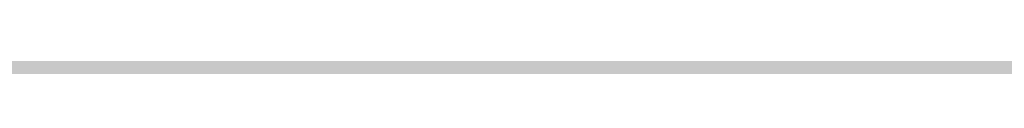
# Model space of a CAD drawing. Units: feet. Extents: x 3168 to 4724, y 827 to 1477.
# Tile 42 of 256: x 3270.273 to 3273.072, y 1099.001 to 1099.015. Entities that reach past the tile are written whole.
import ezdxf

# ---------------------------------------------------------------- set-up
doc = ezdxf.new("R2010")
doc.units = ezdxf.units.FT
doc.layers.add('A-ELEV', color=7, linetype='Continuous', lineweight=35)
doc.layers.add('A-ELEV-PATT', color=8, linetype='Continuous', lineweight=13)

msp = doc.modelspace()

# ---------------------------------------------------------------- hatches: boundary and pattern name
at = {"layer": 'A-ELEV-PATT'}
h = msp.add_hatch(color=256, dxfattribs=at)
h.dxf.hatch_style = 1
edge = h.paths.add_edge_path()
edge.add_ellipse((3552.9058, 979.2201), major_axis=(36.7449, 0), ratio=0.4848485, start_angle=0, end_angle=360)
edge = h.paths.add_edge_path()
edge.add_ellipse((3559.8916, 929.2523), major_axis=(36.7449, 0), ratio=0.4848485, start_angle=0, end_angle=360)
edge = h.paths.add_edge_path()
edge.add_line((3299.3168, 1198.6061), (3479.9167, 1198.6061))
edge.add_line((3479.9167, 1198.6061), (3479.9167, 1209.8686))
edge.add_spline(control_points=[(3479.9167, 1209.8686), (3464.3012, 1209.8686), (3448.6856, 1209.8686), (3410.9491, 1209.8686), (3388.8282, 1209.8686), (3355.6469, 1209.8686), (3344.5864, 1209.8686), (3327.9957, 1209.8686), (3322.4655, 1209.8686), (3314.1702, 1209.8686), (3311.4051, 1209.8686), (3307.2574, 1209.8686), (3305.8748, 1209.8686), (3303.801, 1209.8686), (3303.1097, 1209.8686), (3302.0728, 1209.8686), (3301.7272, 1209.8686), (3301.2087, 1209.8686), (3301.0359, 1209.8686), (3300.7767, 1209.8686), (3300.6903, 1209.8686), (3300.5606, 1209.8686), (3300.5174, 1209.8686), (3300.4526, 1209.8686), (3300.431, 1209.8686), (3300.3986, 1209.8686), (3300.3878, 1209.8686), (3300.3662, 1209.8686), (3300.3457, 1209.8686), (3300.3455, 1209.8686), (3300.3455, 1209.8686), (3300.3433, 1209.8686), (3300.3411, 1209.8686), (3300.3379, 1209.8686), (3300.3368, 1209.8686), (3300.3339, 1209.8686), (3300.3321, 1209.8686), (3300.3255, 1209.8686), (3300.3207, 1209.8686), (3300.3109, 1209.8686), (3300.306, 1209.8686), (3300.2905, 1209.8686), (3300.28, 1209.8686), (3300.2324, 1209.8688), (3300.1953, 1209.869), (3299.9511, 1209.8706), (3299.7448, 1209.8743), (3299.4368, 1209.8833), (3299.3344, 1209.8868), (3299.1811, 1209.8929), (3299.13, 1209.8951), (3298.6522, 1209.9168), (3298.2295, 1209.9457), (3297.6016, 1210.0024), (3297.3934, 1210.0235), (3297.0827, 1210.0583), (3296.9793, 1210.0705), (3296.293, 1210.1549), (3295.7181, 1210.2434), (3294.8687, 1210.3989), (3294.5877, 1210.4545), (3294.1693, 1210.5433), (3294.0304, 1210.5739), (3291.7071, 1211.1012), (3289.6536, 1211.8134), (3285.7763, 1213.564), (3283.9514, 1214.6035), (3280.5122, 1216.9801), (3278.8972, 1218.3176), (3276.3799, 1220.8295), (3275.416, 1221.9177), (3274.0393, 1223.7077), (3273.581, 1224.3495), (3273.1432, 1225.0163)], knot_values=[39.119033, 39.119033, 39.119033, 39.119033, 39.286353, 39.286353, 39.523379, 39.523379, 39.641892, 39.641892, 39.701148, 39.701148, 39.730777, 39.730777, 39.745591, 39.745591, 39.752998, 39.752998, 39.756701, 39.756701, 39.758553, 39.758553, 39.759479, 39.759479, 39.759942, 39.759942, 39.760173, 39.760173, 39.760289, 39.760289, 39.760405, 39.760405, 39.760463, 39.760463, 39.763389, 39.763389, 39.764851, 39.764851, 39.767304, 39.767304, 39.773825, 39.773825, 39.78057, 39.78057, 39.79477, 39.79477, 39.845194, 39.845194, 40.126715, 40.126715, 40.267476, 40.267476, 40.337856, 40.337856, 40.927023, 40.927023, 41.221606, 41.221606, 41.368898, 41.368898, 42.202622, 42.202622, 42.619485, 42.619485, 42.827916, 42.827916, 46.118323, 46.118323, 49.408731, 49.408731, 52.699139, 52.699139, 54.927489, 54.927489, 56.104228, 56.104228, 56.104228, 56.104228], weights=[1, 1, 1, 1, 1, 1, 1, 1, 1, 1, 1, 1, 1, 1, 1, 1, 1, 1, 1, 1, 1, 1, 1, 1, 1, 1, 1, 1, 1, 1, 1, 1, 1, 1, 1, 1, 1, 1, 1, 1, 1, 1, 1, 1, 1, 1, 1, 1, 1, 1, 1, 1, 1, 1, 1, 1, 1, 1, 1, 1, 1, 1, 1, 1, 1, 1, 1, 1, 1, 1, 1, 1, 1, 1], degree=3, periodic=0)
edge.add_line((3273.1432, 1225.0163), (3273.1432, 1099.0163))
edge.add_line((3273.1432, 1099.0163), (3299.3168, 1099.0163))
edge.add_line((3299.3168, 1099.0163), (3299.3168, 1198.6061))
edge = h.paths.add_edge_path()
edge.add_line((3304.7584, 1324.1581), (3479.9167, 1324.1581))
edge.add_line((3479.9167, 1324.1581), (3479.9167, 1335.7146))
edge.add_line((3479.9167, 1335.7146), (3269.1616, 1335.7146))
edge.add_spline(control_points=[(3269.1616, 1335.7146), (3264.0242, 1335.7146), (3258.3641, 1328.9582), (3259.2643, 1323.9003)], knot_values=[0, 0, 0, 0, 15.412191, 15.412191, 15.412191, 15.412191], degree=3, periodic=0)
edge.add_line((3259.2643, 1323.9003), (3265.5168, 1288.7691))
edge.add_line((3265.5168, 1288.7691), (3275.2651, 1261.5456))
edge.add_line((3275.2651, 1261.5456), (3304.7584, 1261.5456))
edge.add_line((3304.7584, 1261.5456), (3304.7584, 1324.1581))
h = msp.add_hatch(color=256, dxfattribs=at)
h.dxf.hatch_style = 1
h.paths.add_polyline_path([(3384.5252, 1099.0163), (3335.0292, 1099.0163), (3299.3168, 1099.0163), (3273.1432, 1099.0163), (3217.5654, 1099.0163), (3168.0693, 827.1163), (3335.0292, 827.1163)])

# ---------------------------------------------------------------- linework, layer by layer
at = {"layer": 'A-ELEV'}
msp.add_open_spline([(3808.5202, 1099.0163), (3808.5202, 1141.4132), (3808.5202, 1183.8102), (3808.5202, 1226.6353), (3808.5202, 1227.0636), (3808.5202, 1227.4918), (3811.4919, 1248.9947), (3814.4635, 1270.4975), (3817.4652, 1292.2176), (3817.4952, 1292.4348), (3817.5253, 1292.652), (3817.5728, 1310.1067), (3817.6203, 1327.5615), (3817.6679, 1345.0163), (3817.6679, 1345.458), (3817.6679, 1345.8996), (3817.6679, 1346.456), (3817.6679, 1346.5708), (3817.6679, 1346.7529), (3817.6679, 1346.8201), (3817.6679, 1346.9349), (3817.6679, 1346.9823), (3817.6679, 1347.0386), (3817.6679, 1347.0474), (3817.6679, 1347.0737), (3817.6679, 1347.0593), (3817.6679, 1347.0615), (3817.6679, 1347.0627), (3817.6679, 1347.066), (3817.6679, 1347.0683), (3817.6679, 1347.075), (3817.6679, 1347.0795), (3817.6678, 1347.0929), (3817.6678, 1347.1019), (3817.6678, 1347.1288), (3817.6677, 1347.1467), (3817.6674, 1347.2004), (3817.6672, 1347.2362), (3817.6661, 1347.3434), (3817.665, 1347.4147), (3817.6608, 1347.6281), (3817.6566, 1347.7697), (3817.64, 1348.1925), (3817.6235, 1348.4716), (3817.5591, 1349.3001), (3817.4961, 1349.8406), (3817.2554, 1351.4242), (3817.0263, 1352.4288), (3816.3069, 1354.8889), (3815.7437, 1356.2687), (3814.464, 1358.8192), (3813.7464, 1359.991), (3812.1958, 1362.1723), (3811.3622, 1363.1821), (3809.5888, 1365.069), (3808.6488, 1365.9461), (3806.6543, 1367.5796), (3805.5997, 1368.3362), (3803.3529, 1369.7223), (3802.1605, 1370.3524), (3799.6008, 1371.4536), (3798.2327, 1371.9255), (3795.2801, 1372.6346), (3793.6931, 1372.8721), (3791.8694, 1372.9265), (3791.7409, 1372.9292), (3791.3534, 1372.9341), (3791.0927, 1372.9329), (3790.3041, 1372.9151), (3789.7695, 1372.8842), (3789.2092, 1372.8302), (3789.1906, 1372.8284), (3789.1349, 1372.8229), (3789.0977, 1372.8191), (3789.0484, 1372.814), (3789.0364, 1372.8127), (3789.0003, 1372.8089), (3788.9761, 1372.8063), (3788.9494, 1372.8034), (3788.9468, 1372.8031), (3788.9426, 1372.8027), (3788.941, 1372.8025), (3788.9386, 1372.8022), (3788.9378, 1372.8021), (3788.9354, 1372.8019), (3788.8675, 1372.7944), (3788.7569, 1372.7822), (3788.7015, 1372.7761), (3788.5355, 1372.7579), (3788.4249, 1372.7457), (3788.0929, 1372.7092), (3787.8715, 1372.6848), (3787.2075, 1372.6118), (3786.7648, 1372.5631), (3785.4368, 1372.417), (3784.5515, 1372.3196), (3781.8954, 1372.0274), (3780.1247, 1371.8327), (3774.8126, 1371.2483), (3771.2713, 1370.8587), (3760.6471, 1369.69), (3753.5643, 1368.9109), (3732.316, 1366.5735), (3718.1504, 1365.0152), (3694.0068, 1362.3593), (3684.0287, 1361.2617), (3674.0506, 1360.1641), (3664.6007, 1360.1641), (3655.1508, 1360.1641), (3626.8011, 1360.1641), (3607.9013, 1360.1641), (3551.2019, 1360.1641), (3513.4023, 1360.1641), (3467.7252, 1360.1641), (3459.8476, 1360.1641), (3436.2149, 1360.1641), (3420.4597, 1360.1641), (3373.1943, 1360.1641), (3341.6839, 1360.1641), (3302.8482, 1360.1641), (3295.5227, 1360.1641), (3286.0383, 1360.1641), (3283.8794, 1360.1641), (3277.4026, 1360.1641), (3273.0848, 1360.1641), (3267.7329, 1360.1641), (3266.6988, 1360.1641), (3263.5965, 1360.1641), (3261.5284, 1360.1641), (3259.2369, 1360.1641), (3259.0137, 1360.1641), (3258.344, 1360.1641), (3257.8975, 1360.1641), (3257.431, 1360.1641), (3257.411, 1360.1641), (3257.3706, 1360.1641), (3257.3755, 1360.1641), (3257.3746, 1360.1641), (3257.3739, 1360.1641), (3257.372, 1360.1641), (3257.3706, 1360.1641), (3257.3667, 1360.1641), (3257.364, 1360.1641), (3257.3561, 1360.1641), (3257.3508, 1360.164), (3257.335, 1360.164), (3257.3244, 1360.164), (3257.2928, 1360.1639), (3257.2717, 1360.1638), (3257.2084, 1360.1634), (3257.1663, 1360.163), (3257.0402, 1360.1614), (3256.9563, 1360.1598), (3256.7055, 1360.1534), (3256.5392, 1360.147), (3256.0436, 1360.1219), (3255.7173, 1360.0971), (3254.7524, 1360.0005), (3254.128, 1359.9065), (3252.1801, 1359.5253), (3250.9416, 1359.144), (3248.6702, 1358.2433), (3247.6357, 1357.7238), (3245.7326, 1356.6035), (3244.8634, 1356.0021), (3243.2531, 1354.7429), (3242.512, 1354.0847), (3240.7511, 1352.3448), (3239.801, 1351.2296), (3238.0878, 1348.8724), (3237.3247, 1347.6304), (3235.9825, 1344.9716), (3235.4022, 1343.5549), (3234.5911, 1340.8155), (3234.3109, 1339.5435), (3233.9765, 1336.8026), (3233.9221, 1335.3309), (3234.1489, 1332.5913), (3234.3495, 1331.3672), (3234.7199, 1329.9994), (3234.7524, 1329.8834), (3234.8536, 1329.5348), (3234.9259, 1329.3017), (3235.0248, 1329.0026), (3235.0469, 1328.9369), (3235.0776, 1328.8472), (3235.0859, 1328.8232), (3235.1109, 1328.7511), (3235.1278, 1328.703), (3235.148, 1328.6462), (3235.1511, 1328.6376), (3235.1561, 1328.6235), (3235.1581, 1328.618), (3235.1602, 1328.612), (3235.1656, 1328.5969), (3235.1801, 1328.5565), (3235.1903, 1328.5281), (3235.2208, 1328.4429), (3235.2411, 1328.3862), (3235.3021, 1328.2159), (3235.3427, 1328.1023), (3235.4647, 1327.7617), (3235.546, 1327.5346), (3235.79, 1326.8534), (3235.9526, 1326.3992), (3236.4405, 1325.0367), (3236.7657, 1324.1284), (3237.7415, 1321.4034), (3238.392, 1319.5868), (3240.3435, 1314.1369), (3241.6445, 1310.5036), (3245.5476, 1299.6037), (3248.1496, 1292.3371), (3255.9557, 1270.5374), (3261.1598, 1256.0042), (3267.3876, 1238.612), (3268.4114, 1235.7529), (3269.5104, 1232.6839), (3269.5856, 1232.4739), (3269.7066, 1232.1359), (3269.7524, 1232.0079), (3269.8273, 1231.7987), (3269.8564, 1231.7176), (3269.9063, 1231.5781), (3269.9272, 1231.5198), (3269.9725, 1231.3934), (3269.9968, 1231.3254), (3270.0265, 1231.2425), (3270.0318, 1231.2277), (3270.0403, 1231.204), (3270.0392, 1231.207), (3270.0394, 1231.2066), (3270.0394, 1231.2064), (3270.0396, 1231.2058), (3270.0398, 1231.2055), (3270.0402, 1231.2043), (3270.0404, 1231.2036), (3270.0413, 1231.2013), (3270.0418, 1231.1998), (3270.0434, 1231.1953), (3270.0445, 1231.1922), (3270.0478, 1231.1832), (3270.0499, 1231.1771), (3270.0564, 1231.159), (3270.0608, 1231.147), (3270.0739, 1231.1108), (3270.0826, 1231.0867), (3270.1089, 1231.0144), (3270.1266, 1230.9663), (3270.1799, 1230.8225), (3270.2159, 1230.7269), (3270.3253, 1230.4415), (3270.4, 1230.2528), (3270.6292, 1229.6914), (3270.7889, 1229.3235), (3271.2865, 1228.2383), (3271.6431, 1227.5398), (3272.7759, 1225.5153), (3273.6142, 1224.2605), (3275.416, 1221.9177), (3276.3799, 1220.8295), (3278.8972, 1218.3176), (3280.5122, 1216.9801), (3283.9514, 1214.6035), (3285.7763, 1213.564), (3289.6536, 1211.8134), (3291.7071, 1211.1012), (3294.0304, 1210.5739), (3294.1693, 1210.5433), (3294.5877, 1210.4545), (3294.8687, 1210.3989), (3295.7181, 1210.2434), (3296.293, 1210.1549), (3296.9793, 1210.0705), (3297.0827, 1210.0583), (3297.3934, 1210.0235), (3297.6016, 1210.0024), (3298.2295, 1209.9457), (3298.6522, 1209.9168), (3299.13, 1209.8951), (3299.1811, 1209.8929), (3299.3344, 1209.8868), (3299.4368, 1209.8833), (3299.7448, 1209.8743), (3299.9511, 1209.8706), (3300.1953, 1209.869), (3300.2324, 1209.8688), (3300.28, 1209.8686), (3300.2905, 1209.8686), (3300.306, 1209.8686), (3300.3109, 1209.8686), (3300.3207, 1209.8686), (3300.3255, 1209.8686), (3300.3321, 1209.8686), (3300.3339, 1209.8686), (3300.3368, 1209.8686), (3300.3379, 1209.8686), (3300.3411, 1209.8686), (3300.3433, 1209.8686), (3300.3455, 1209.8686), (3300.3455, 1209.8686), (3300.3457, 1209.8686), (3300.3662, 1209.8686), (3300.3878, 1209.8686), (3300.3986, 1209.8686), (3300.431, 1209.8686), (3300.4526, 1209.8686), (3300.5174, 1209.8686), (3300.5606, 1209.8686), (3300.6903, 1209.8686), (3300.7767, 1209.8686), (3301.0359, 1209.8686), (3301.2087, 1209.8686), (3301.7272, 1209.8686), (3302.0728, 1209.8686), (3303.1097, 1209.8686), (3303.801, 1209.8686), (3305.8748, 1209.8686), (3307.2574, 1209.8686), (3311.4051, 1209.8686), (3314.1702, 1209.8686), (3322.4655, 1209.8686), (3327.9957, 1209.8686), (3344.5864, 1209.8686), (3355.6469, 1209.8686), (3388.8282, 1209.8686), (3410.9491, 1209.8686), (3477.3119, 1209.8686), (3521.5537, 1209.8686), (3566.8362, 1209.8686), (3567.8769, 1209.8686), (3570.999, 1209.8686), (3573.0804, 1209.8686), (3575.7814, 1209.8686), (3576.4009, 1209.8686), (3577.2958, 1209.8686), (3577.5712, 1209.8686), (3578.3971, 1209.8686), (3578.9478, 1209.8686), (3579.7565, 1209.8686), (3580.0145, 1209.8686), (3580.3427, 1209.8686), (3580.3269, 1209.8686), (3580.3272, 1209.8686), (3580.3273, 1209.8686), (3580.3278, 1209.8686), (3580.3281, 1209.8686), (3580.329, 1209.8686), (3580.3296, 1209.8686), (3580.3314, 1209.8686), (3580.3327, 1209.8686), (3580.3363, 1209.8686), (3580.3388, 1209.8686), (3580.3461, 1209.8686), (3580.351, 1209.8686), (3580.3657, 1209.8685), (3580.3754, 1209.8685), (3580.4048, 1209.8684), (3580.4244, 1209.8684), (3580.4832, 1209.8681), (3580.5224, 1209.8678), (3580.6404, 1209.8666), (3580.7192, 1209.8655), (3580.9563, 1209.8608), (3581.1152, 1209.8561), (3581.5942, 1209.8372), (3581.9164, 1209.8183), (3582.8899, 1209.7424), (3583.548, 1209.6662), (3585.5318, 1209.3606), (3586.8672, 1209.0539), (3589.4715, 1208.2525), (3590.7402, 1207.7579), (3591.9955, 1207.1588), (3592.0578, 1207.1287), (3592.2442, 1207.038), (3592.3677, 1206.9766), (3592.7353, 1206.7904), (3592.9768, 1206.6631), (3593.2445, 1206.5164), (3593.2747, 1206.4998), (3593.3651, 1206.4498), (3593.4251, 1206.4163), (3593.6043, 1206.3153), (3593.7227, 1206.2472), (3593.8572, 1206.1684), (3593.8744, 1206.1583), (3593.9257, 1206.128), (3593.9599, 1206.1078), (3594.0621, 1206.0469), (3594.1298, 1206.0061), (3594.2084, 1205.9582), (3594.2197, 1205.9513), (3594.2534, 1205.9307), (3594.2758, 1205.9169), (3594.343, 1205.8755), (3594.3876, 1205.8479), (3594.4336, 1205.819), (3594.4353, 1205.818), (3594.4402, 1205.8149), (3594.4435, 1205.8129), (3594.4471, 1205.8106), (3594.4475, 1205.8103), (3594.4487, 1205.8096), (3594.4495, 1205.8091), (3594.4504, 1205.8086), (3594.4505, 1205.8085), (3594.4506, 1205.8084), (3594.4674, 1205.7979), (3594.4933, 1205.7817), (3594.5062, 1205.7736), (3594.545, 1205.7492), (3594.5709, 1205.733), (3594.6485, 1205.6844), (3594.7002, 1205.652), (3594.8554, 1205.5547), (3594.9589, 1205.4898), (3595.2694, 1205.2953), (3595.4763, 1205.1656), (3596.0972, 1204.7765), (3596.5111, 1204.5171), (3597.7528, 1203.7388), (3598.5807, 1203.22), (3601.0642, 1201.6636), (3602.7198, 1200.6259), (3607.6868, 1197.513), (3610.9981, 1195.4377), (3620.932, 1189.2119), (3627.5546, 1185.0614), (3647.4225, 1172.6097), (3660.6678, 1164.3086), (3700.4035, 1139.4053), (3726.894, 1122.8031), (3757.2057, 1103.8061), (3761.027, 1101.4112), (3764.8482, 1099.0163), (3745.3283, 1099.0163), (3725.8083, 1099.0163), (3706.2884, 1099.0163), (3706.2884, 1108.4532), (3706.2884, 1117.8902), (3706.2884, 1127.3271), (3710.7508, 1127.3271), (3715.2131, 1127.3271), (3719.6755, 1127.3271)], degree=3, knots=[0, 0, 0, 0, 0.982037, 0.982037, 0.991957, 0.991957, 0.991957, 1.966522, 1.966522, 1.976367, 1.976367, 1.976367, 2.976367, 2.976367, 2.976367, 3.00169, 3.00169, 3.008272, 3.008272, 3.012129, 3.012129, 3.014851, 3.014851, 3.015353, 3.015353, 3.016359, 3.016359, 3.017365, 3.017365, 3.019376, 3.019376, 3.023398, 3.023398, 3.031442, 3.031442, 3.047531, 3.047531, 3.079708, 3.079708, 3.144063, 3.144063, 3.272772, 3.272772, 3.53019, 3.53019, 4.045026, 4.045026, 5.074698, 5.074698, 6.700878, 6.700878, 8.327058, 8.327058, 9.953238, 9.953238, 11.579418, 11.579418, 13.205598, 13.205598, 14.831778, 14.831778, 16.457958, 16.457958, 18.084138, 18.084138, 18.206872, 18.206872, 18.45234, 18.45234, 18.943275, 18.943275, 18.960093, 18.960093, 18.993729, 18.993729, 19.00461, 19.00461, 19.026374, 19.026374, 19.028737, 19.028737, 19.03018, 19.03018, 19.030897, 19.030897, 19.032332, 19.032332, 19.033766, 19.033766, 19.036636, 19.036636, 19.042374, 19.042374, 19.053851, 19.053851, 19.076805, 19.076805, 19.122714, 19.122714, 19.21453, 19.21453, 19.398163, 19.398163, 19.765429, 19.765429, 20.024128, 20.024128, 20.024128, 20.092031, 20.092031, 20.227836, 20.227836, 20.499446, 20.499446, 20.556051, 20.556051, 20.66926, 20.66926, 20.895678, 20.895678, 20.948316, 20.948316, 20.963829, 20.963829, 20.994855, 20.994855, 21.002285, 21.002285, 21.017146, 21.017146, 21.01875, 21.01875, 21.021959, 21.021959, 21.022102, 21.022102, 21.022249, 21.022249, 21.022708, 21.022708, 21.023627, 21.023627, 21.025464, 21.025464, 21.029138, 21.029138, 21.036486, 21.036486, 21.051183, 21.051183, 21.080575, 21.080575, 21.139361, 21.139361, 21.256932, 21.256932, 21.492073, 21.492073, 21.962356, 21.962356, 23.01002, 23.01002, 24.057684, 24.057684, 25.105348, 25.105348, 26.153011, 26.153011, 27.776787, 27.776787, 29.400562, 29.400562, 31.024337, 31.024337, 32.278801, 32.278801, 33.533265, 33.533265, 34.467568, 34.467568, 34.553971, 34.553971, 34.726776, 34.726776, 34.775309, 34.775309, 34.793079, 34.793079, 34.82862, 34.82862, 34.834979, 34.834979, 34.839039, 34.839039, 34.839411, 34.839411, 34.840285, 34.840285, 34.842034, 34.842034, 34.845531, 34.845531, 34.852525, 34.852525, 34.866512, 34.866512, 34.894488, 34.894488, 34.950439, 34.950439, 35.062342, 35.062342, 35.286147, 35.286147, 35.733758, 35.733758, 35.821815, 35.821815, 35.828283, 35.828283, 35.832225, 35.832225, 35.834724, 35.834724, 35.836521, 35.836521, 35.838617, 35.838617, 35.839073, 35.839073, 35.839345, 35.839345, 35.839617, 35.839617, 35.840161, 35.840161, 35.841249, 35.841249, 35.843425, 35.843425, 35.847778, 35.847778, 35.856482, 35.856482, 35.873891, 35.873891, 35.908709, 35.908709, 35.978345, 35.978345, 36.117617, 36.117617, 36.396161, 36.396161, 36.953248, 36.953248, 38.067423, 38.067423, 40.295772, 40.295772, 42.524122, 42.524122, 45.81453, 45.81453, 49.104937, 49.104937, 52.395345, 52.395345, 52.603776, 52.603776, 53.020639, 53.020639, 53.854363, 53.854363, 54.001655, 54.001655, 54.296238, 54.296238, 54.885405, 54.885405, 54.955785, 54.955785, 55.096546, 55.096546, 55.378067, 55.378067, 55.42849, 55.42849, 55.442691, 55.442691, 55.449436, 55.449436, 55.455957, 55.455957, 55.458409, 55.458409, 55.459872, 55.459872, 55.462798, 55.462798, 55.462856, 55.462856, 55.462972, 55.462972, 55.463088, 55.463088, 55.463319, 55.463319, 55.463782, 55.463782, 55.464708, 55.464708, 55.46656, 55.46656, 55.470263, 55.470263, 55.47767, 55.47767, 55.492484, 55.492484, 55.522112, 55.522112, 55.581369, 55.581369, 55.699882, 55.699882, 55.936907, 55.936907, 56.410959, 56.410959, 56.42211, 56.42211, 56.444413, 56.444413, 56.451051, 56.451051, 56.454001, 56.454001, 56.459901, 56.459901, 56.462666, 56.462666, 56.463418, 56.463418, 56.464171, 56.464171, 56.465675, 56.465675, 56.468684, 56.468684, 56.474702, 56.474702, 56.486738, 56.486738, 56.51081, 56.51081, 56.558955, 56.558955, 56.655243, 56.655243, 56.847821, 56.847821, 57.232975, 57.232975, 58.003284, 58.003284, 59.543901, 59.543901, 62.625137, 62.625137, 68.787607, 68.787607, 74.950078, 74.950078, 75.27336, 75.27336, 75.919923, 75.919923, 77.213051, 77.213051, 77.377769, 77.377769, 77.707206, 77.707206, 78.366079, 78.366079, 78.462532, 78.462532, 78.655436, 78.655436, 79.041245, 79.041245, 79.105735, 79.105735, 79.234714, 79.234714, 79.492672, 79.492672, 79.502197, 79.502197, 79.521249, 79.521249, 79.523534, 79.523534, 79.528103, 79.528103, 79.528682, 79.528682, 79.528885, 79.528885, 79.529089, 79.529089, 79.529495, 79.529495, 79.530308, 79.530308, 79.531935, 79.531935, 79.535187, 79.535187, 79.541693, 79.541693, 79.554704, 79.554704, 79.580725, 79.580725, 79.632769, 79.632769, 79.736856, 79.736856, 79.94503, 79.94503, 80.361377, 80.361377, 80.421435, 80.421435, 80.421435, 81.421435, 81.421435, 81.421435, 82.421435, 82.421435, 82.421435, 83.421435, 83.421435, 83.421435, 83.421435], dxfattribs=at)

doc.saveas('drawing.dxf')
